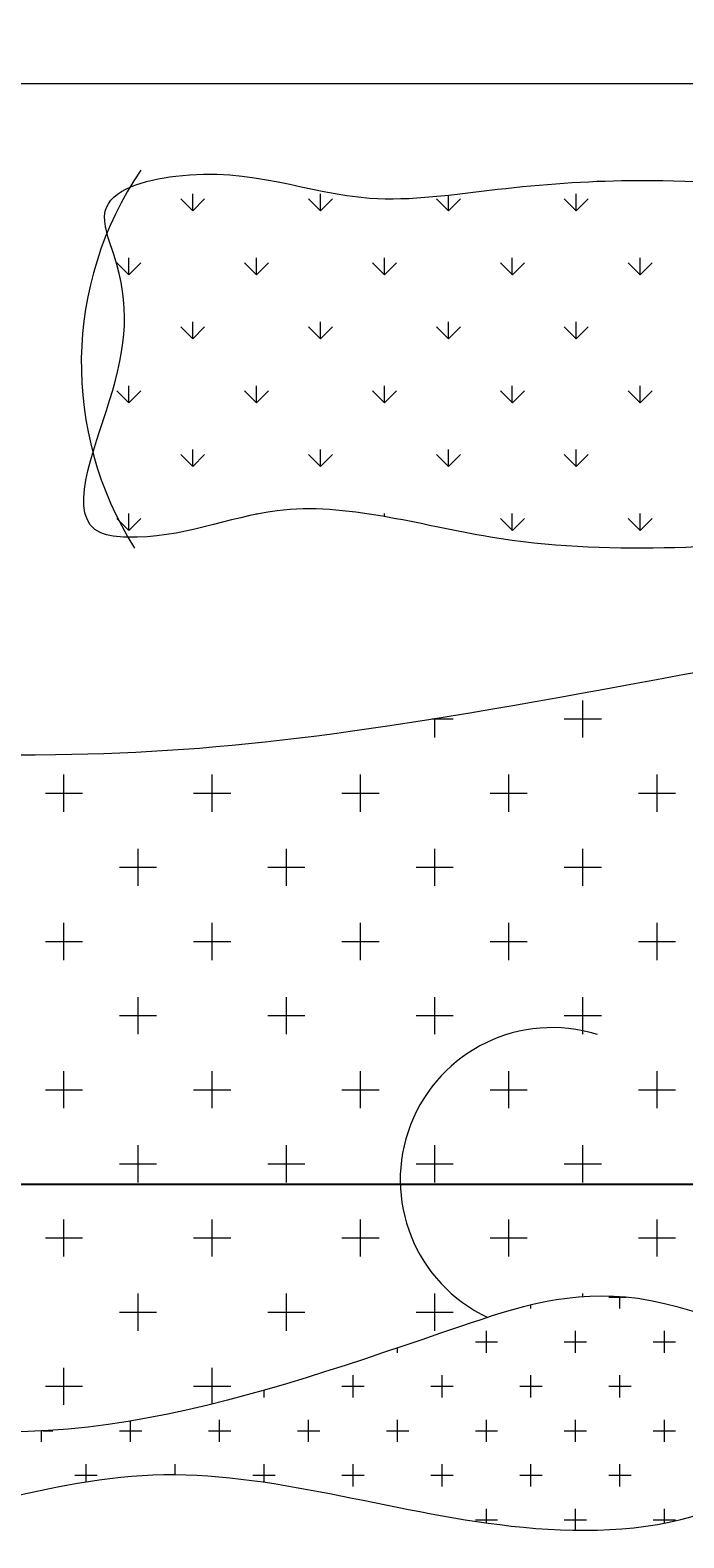
# Model space of a CAD drawing. Units: inches. Extents: x 2330 to 3943, y 1763 to 3461.
# Tile 6 of 40: x 2564 to 2593, y 2316 to 2383. Entities that reach past the tile are written whole.
import ezdxf

# ---------------------------------------------------------------- set-up
doc = ezdxf.new("R2010")
doc.units = ezdxf.units.IN
doc.layers.add('A-ANNO-DIMS', color=2, linetype='Continuous', lineweight=18)
doc.layers.add('A-FURN', color=8, linetype='Continuous', lineweight=13)
doc.styles.get("Standard").update_dxf_attribs({"font": 'arial.ttf'})
doc.dimstyles.get("Standard").update_dxf_attribs({"dimtxt": 0.18, "dimasz": 0.18, "dimexe": 0.18, "dimexo": 0.0625, "dimgap": 0.09, "dimtad": 0, "dimtih": 1, "dimtoh": 1, "dimdec": 4, "dimzin": 0, "dimdsep": 46, "dimtxsty": 'Standard', "dimcen": 0.09, "dimadec": 0, "dimazin": 0, "dimtfac": 1, "dimtdec": 4, "dimtofl": 0, "dimtmove": 0, "dimatfit": 3, "dimfxl": 1, "dimtolj": 1, "dimtzin": 0, "dimarcsym": 0})

# ---------------------------------------------------------------- blocks, each defined once
blk = doc.blocks.new('A$C200C7901')
for p, q in [((0.5, 2.3334), (2, 2.3334)), ((1.3176, 2.1721), (1.3075, 2.1822)), ((1.3176, 2.1721), (1.3075, 2.1822))]:
    blk.add_line(p, q)
at = {"linetype": 'ByBlock'}
for p, q in [((1.3714, 2.2259), (1.3714, 2.2402)), ((1.3714, 2.2259), (1.3714, 2.2402)), ((1.4792, 2.2259), (1.4792, 2.2402)), ((1.4792, 2.2259), (1.4792, 2.2402)), ((1.587, 2.2259), (1.587, 2.2393)), ((1.587, 2.2259), (1.587, 2.2393)), ((1.6947, 2.2259), (1.6947, 2.2402)), ((1.6947, 2.2259), (1.6947, 2.2402)), ((1.3714, 2.2259), (1.3613, 2.236)), ((1.3714, 2.2259), (1.3613, 2.236)), ((1.3714, 2.2259), (1.3815, 2.236)), ((1.3714, 2.2259), (1.3815, 2.236)), ((1.4792, 2.2259), (1.4691, 2.236)), ((1.4792, 2.2259), (1.4691, 2.236)), ((1.4792, 2.2259), (1.4893, 2.236)), ((1.4792, 2.2259), (1.4893, 2.236)), ((1.587, 2.2259), (1.5769, 2.236)), ((1.587, 2.2259), (1.5769, 2.236)), ((1.587, 2.2259), (1.5971, 2.236)), ((1.587, 2.2259), (1.5971, 2.236)), ((1.6947, 2.2259), (1.6846, 2.236)), ((1.6947, 2.2259), (1.6846, 2.236)), ((1.6947, 2.2259), (1.7048, 2.236)), ((1.6947, 2.2259), (1.7048, 2.236)), ((1.3176, 2.172), (1.3176, 2.1863)), ((1.3176, 2.172), (1.3176, 2.1863)), ((1.4253, 2.172), (1.4253, 2.1863)), ((1.4253, 2.172), (1.4253, 2.1863)), ((1.5331, 2.172), (1.5331, 2.1863)), ((1.5331, 2.172), (1.5331, 2.1863)), ((1.6408, 2.172), (1.6408, 2.1863)), ((1.6408, 2.172), (1.6408, 2.1863)), ((1.7486, 2.172), (1.7486, 2.1863)), ((1.7486, 2.172), (1.7486, 2.1863)), ((1.3176, 2.1721), (1.3277, 2.1822)), ((1.3176, 2.1721), (1.3277, 2.1822)), ((1.4253, 2.1721), (1.4152, 2.1822)), ((1.4253, 2.1721), (1.4152, 2.1822)), ((1.4253, 2.1721), (1.4354, 2.1822)), ((1.4253, 2.1721), (1.4354, 2.1822)), ((1.5331, 2.1721), (1.523, 2.1822)), ((1.5331, 2.1721), (1.523, 2.1822)), ((1.5331, 2.1721), (1.5432, 2.1822)), ((1.5331, 2.1721), (1.5432, 2.1822)), ((1.6409, 2.1721), (1.6308, 2.1822)), ((1.6409, 2.1721), (1.6308, 2.1822)), ((1.6409, 2.1721), (1.651, 2.1822)), ((1.6409, 2.1721), (1.651, 2.1822)), ((1.7486, 2.1721), (1.7385, 2.1822)), ((1.7486, 2.1721), (1.7385, 2.1822)), ((1.7486, 2.1721), (1.7587, 2.1822)), ((1.7486, 2.1721), (1.7587, 2.1822)), ((1.3714, 2.1182), (1.3613, 2.1283)), ((1.3714, 2.1182), (1.3613, 2.1283)), ((1.3714, 2.1182), (1.3714, 2.1325)), ((1.3714, 2.1182), (1.3714, 2.1325)), ((1.3714, 2.1182), (1.3815, 2.1283)), ((1.3714, 2.1182), (1.3815, 2.1283)), ((1.4792, 2.1182), (1.4691, 2.1283)), ((1.4792, 2.1182), (1.4691, 2.1283)), ((1.4792, 2.1182), (1.4792, 2.1325)), ((1.4792, 2.1182), (1.4792, 2.1325)), ((1.4792, 2.1182), (1.4893, 2.1283)), ((1.4792, 2.1182), (1.4893, 2.1283)), ((1.587, 2.1182), (1.5769, 2.1283)), ((1.587, 2.1182), (1.5769, 2.1283)), ((1.587, 2.1182), (1.587, 2.1325)), ((1.587, 2.1182), (1.587, 2.1325)), ((1.587, 2.1182), (1.5971, 2.1283)), ((1.587, 2.1182), (1.5971, 2.1283)), ((1.6947, 2.1182), (1.6846, 2.1283)), ((1.6947, 2.1182), (1.6846, 2.1283)), ((1.6947, 2.1182), (1.6947, 2.1325)), ((1.6947, 2.1182), (1.6947, 2.1325)), ((1.6947, 2.1182), (1.7048, 2.1283)), ((1.6947, 2.1182), (1.7048, 2.1283)), ((1.3176, 2.0643), (1.3075, 2.0744)), ((1.3176, 2.0643), (1.3075, 2.0744)), ((1.3176, 2.0643), (1.3176, 2.0786)), ((1.3176, 2.0643), (1.3176, 2.0786)), ((1.3176, 2.0643), (1.3277, 2.0744)), ((1.3176, 2.0643), (1.3277, 2.0744)), ((1.4253, 2.0643), (1.4152, 2.0744)), ((1.4253, 2.0643), (1.4152, 2.0744)), ((1.4253, 2.0643), (1.4253, 2.0786)), ((1.4253, 2.0643), (1.4253, 2.0786)), ((1.4253, 2.0643), (1.4354, 2.0744)), ((1.4253, 2.0643), (1.4354, 2.0744)), ((1.5331, 2.0643), (1.523, 2.0744)), ((1.5331, 2.0643), (1.523, 2.0744)), ((1.5331, 2.0643), (1.5331, 2.0786)), ((1.5331, 2.0643), (1.5331, 2.0786)), ((1.5331, 2.0643), (1.5432, 2.0744)), ((1.5331, 2.0643), (1.5432, 2.0744)), ((1.6409, 2.0643), (1.6308, 2.0744)), ((1.6409, 2.0643), (1.6308, 2.0744)), ((1.6408, 2.0643), (1.6408, 2.0786)), ((1.6408, 2.0643), (1.6408, 2.0786)), ((1.6409, 2.0643), (1.651, 2.0744)), ((1.6409, 2.0643), (1.651, 2.0744)), ((1.7486, 2.0643), (1.7385, 2.0744)), ((1.7486, 2.0643), (1.7385, 2.0744)), ((1.7486, 2.0643), (1.7486, 2.0786)), ((1.7486, 2.0643), (1.7486, 2.0786)), ((1.7486, 2.0643), (1.7587, 2.0744)), ((1.7486, 2.0643), (1.7587, 2.0744)), ((1.3714, 2.0104), (1.3714, 2.0247)), ((1.3714, 2.0104), (1.3714, 2.0247)), ((1.4792, 2.0104), (1.4792, 2.0247)), ((1.4792, 2.0104), (1.4792, 2.0247)), ((1.587, 2.0104), (1.587, 2.0247)), ((1.587, 2.0104), (1.587, 2.0247)), ((1.6947, 2.0104), (1.6947, 2.0247)), ((1.6947, 2.0104), (1.6947, 2.0247)), ((1.3714, 2.0104), (1.3613, 2.0205)), ((1.3714, 2.0104), (1.3613, 2.0205)), ((1.3714, 2.0104), (1.3815, 2.0205)), ((1.3714, 2.0104), (1.3815, 2.0205)), ((1.4792, 2.0104), (1.4691, 2.0205)), ((1.4792, 2.0104), (1.4691, 2.0205)), ((1.4792, 2.0104), (1.4893, 2.0205)), ((1.4792, 2.0104), (1.4893, 2.0205)), ((1.587, 2.0104), (1.5769, 2.0205)), ((1.587, 2.0104), (1.5769, 2.0205)), ((1.587, 2.0104), (1.5971, 2.0205)), ((1.587, 2.0104), (1.5971, 2.0205)), ((1.6947, 2.0104), (1.6846, 2.0205)), ((1.6947, 2.0104), (1.6846, 2.0205)), ((1.6947, 2.0104), (1.7048, 2.0205)), ((1.6947, 2.0104), (1.7048, 2.0205)), ((1.3176, 1.9565), (1.3176, 1.9708)), ((1.3176, 1.9565), (1.3176, 1.9708)), ((1.4253, 1.9703), (1.4253, 1.9708)), ((1.4253, 1.9703), (1.4253, 1.9708)), ((1.5331, 1.9683), (1.5331, 1.9708)), ((1.5331, 1.9683), (1.5331, 1.9708)), ((1.6408, 1.9565), (1.6408, 1.9708)), ((1.6408, 1.9565), (1.6408, 1.9708)), ((1.7486, 1.9565), (1.7486, 1.9708)), ((1.7486, 1.9565), (1.7486, 1.9708)), ((1.3176, 1.9565), (1.3075, 1.9666)), ((1.3176, 1.9565), (1.3075, 1.9666)), ((1.3176, 1.9565), (1.3277, 1.9666)), ((1.3176, 1.9565), (1.3277, 1.9666)), ((1.543, 1.9665), (1.5432, 1.9666)), ((1.543, 1.9665), (1.5432, 1.9666)), ((1.6409, 1.9565), (1.6308, 1.9666)), ((1.6409, 1.9565), (1.6308, 1.9666)), ((1.6409, 1.9565), (1.651, 1.9666)), ((1.6409, 1.9565), (1.651, 1.9666)), ((1.7486, 1.9565), (1.7385, 1.9666)), ((1.7486, 1.9565), (1.7385, 1.9666)), ((1.7486, 1.9565), (1.7587, 1.9666)), ((1.7486, 1.9565), (1.7587, 1.9666)), ((1.7004, 1.782), (1.7004, 1.8133)), ((1.7004, 1.782), (1.7004, 1.8133)), ((1.573, 1.7977), (1.591, 1.7977)), ((1.573, 1.7977), (1.591, 1.7977)), ((1.5754, 1.782), (1.5754, 1.7981)), ((1.5754, 1.782), (1.5754, 1.7981)), ((1.6847, 1.7977), (1.716, 1.7977)), ((1.6847, 1.7977), (1.716, 1.7977)), ((1.2629, 1.7195), (1.2629, 1.7508)), ((1.2629, 1.7195), (1.2629, 1.7508)), ((1.3879, 1.7195), (1.3879, 1.7508)), ((1.3879, 1.7195), (1.3879, 1.7508)), ((1.5129, 1.7195), (1.5129, 1.7508)), ((1.5129, 1.7195), (1.5129, 1.7508)), ((1.6379, 1.7195), (1.6379, 1.7508)), ((1.6379, 1.7195), (1.6379, 1.7508)), ((1.7629, 1.7195), (1.7629, 1.7508)), ((1.7629, 1.7195), (1.7629, 1.7508)), ((1.2472, 1.7352), (1.2785, 1.7352)), ((1.2472, 1.7352), (1.2785, 1.7352)), ((1.3722, 1.7352), (1.4035, 1.7352)), ((1.3722, 1.7352), (1.4035, 1.7352)), ((1.4972, 1.7352), (1.5285, 1.7352)), ((1.4972, 1.7352), (1.5285, 1.7352)), ((1.6222, 1.7352), (1.6535, 1.7352)), ((1.6222, 1.7352), (1.6535, 1.7352)), ((1.7472, 1.7352), (1.7785, 1.7352)), ((1.7472, 1.7352), (1.7785, 1.7352)), ((1.3254, 1.657), (1.3254, 1.6883)), ((1.3254, 1.657), (1.3254, 1.6883)), ((1.4504, 1.657), (1.4504, 1.6883)), ((1.4504, 1.657), (1.4504, 1.6883)), ((1.5754, 1.657), (1.5754, 1.6883)), ((1.5754, 1.657), (1.5754, 1.6883)), ((1.7004, 1.657), (1.7004, 1.6883)), ((1.7004, 1.657), (1.7004, 1.6883)), ((1.3097, 1.6727), (1.341, 1.6727)), ((1.3097, 1.6727), (1.341, 1.6727)), ((1.4347, 1.6727), (1.466, 1.6727)), ((1.4347, 1.6727), (1.466, 1.6727)), ((1.5597, 1.6727), (1.591, 1.6727)), ((1.5597, 1.6727), (1.591, 1.6727)), ((1.6847, 1.6727), (1.716, 1.6727)), ((1.6847, 1.6727), (1.716, 1.6727)), ((1.2629, 1.5945), (1.2629, 1.6258)), ((1.2629, 1.5945), (1.2629, 1.6258)), ((1.3879, 1.5945), (1.3879, 1.6258)), ((1.3879, 1.5945), (1.3879, 1.6258)), ((1.5129, 1.5945), (1.5129, 1.6258)), ((1.5129, 1.5945), (1.5129, 1.6258)), ((1.6379, 1.5945), (1.6379, 1.6258)), ((1.6379, 1.5945), (1.6379, 1.6258)), ((1.7629, 1.5945), (1.7629, 1.6258)), ((1.7629, 1.5945), (1.7629, 1.6258)), ((1.2472, 1.6102), (1.2785, 1.6102)), ((1.2472, 1.6102), (1.2785, 1.6102)), ((1.3722, 1.6102), (1.4035, 1.6102)), ((1.3722, 1.6102), (1.4035, 1.6102)), ((1.4972, 1.6102), (1.5285, 1.6102)), ((1.4972, 1.6102), (1.5285, 1.6102)), ((1.6222, 1.6102), (1.6535, 1.6102)), ((1.6222, 1.6102), (1.6535, 1.6102)), ((1.7472, 1.6102), (1.7785, 1.6102)), ((1.7472, 1.6102), (1.7785, 1.6102)), ((1.3254, 1.532), (1.3254, 1.5633)), ((1.3254, 1.532), (1.3254, 1.5633)), ((1.4504, 1.532), (1.4504, 1.5633)), ((1.4504, 1.532), (1.4504, 1.5633)), ((1.5754, 1.532), (1.5754, 1.5633)), ((1.5754, 1.532), (1.5754, 1.5633)), ((1.7004, 1.532), (1.7004, 1.5633)), ((1.7004, 1.532), (1.7004, 1.5633)), ((1.3097, 1.5477), (1.341, 1.5477)), ((1.3097, 1.5477), (1.341, 1.5477)), ((1.4347, 1.5477), (1.466, 1.5477)), ((1.4347, 1.5477), (1.466, 1.5477)), ((1.5597, 1.5477), (1.591, 1.5477)), ((1.5597, 1.5477), (1.591, 1.5477)), ((1.6847, 1.5477), (1.716, 1.5477)), ((1.6847, 1.5477), (1.716, 1.5477)), ((1.2629, 1.4695), (1.2629, 1.5008)), ((1.2629, 1.4695), (1.2629, 1.5008)), ((1.3879, 1.4695), (1.3879, 1.5008)), ((1.3879, 1.4695), (1.3879, 1.5008)), ((1.5129, 1.4695), (1.5129, 1.5008)), ((1.5129, 1.4695), (1.5129, 1.5008)), ((1.6379, 1.4695), (1.6379, 1.5008)), ((1.6379, 1.4695), (1.6379, 1.5008)), ((1.7629, 1.4695), (1.7629, 1.5008)), ((1.7629, 1.4695), (1.7629, 1.5008)), ((1.2472, 1.4852), (1.2785, 1.4852)), ((1.2472, 1.4852), (1.2785, 1.4852)), ((1.3722, 1.4852), (1.4035, 1.4852)), ((1.3722, 1.4852), (1.4035, 1.4852)), ((1.4972, 1.4852), (1.5285, 1.4852)), ((1.4972, 1.4852), (1.5285, 1.4852)), ((1.6222, 1.4852), (1.6535, 1.4852)), ((1.6222, 1.4852), (1.6535, 1.4852)), ((1.7472, 1.4852), (1.7785, 1.4852)), ((1.7472, 1.4852), (1.7785, 1.4852)), ((1.3254, 1.407), (1.3254, 1.4383)), ((1.3254, 1.407), (1.3254, 1.4383)), ((1.4504, 1.407), (1.4504, 1.4383)), ((1.4504, 1.407), (1.4504, 1.4383)), ((1.5754, 1.407), (1.5754, 1.4383)), ((1.5754, 1.407), (1.5754, 1.4383)), ((1.7004, 1.407), (1.7004, 1.4383)), ((1.7004, 1.407), (1.7004, 1.4383)), ((1.3097, 1.4227), (1.341, 1.4227)), ((1.3097, 1.4227), (1.341, 1.4227)), ((1.4347, 1.4227), (1.466, 1.4227)), ((1.4347, 1.4227), (1.466, 1.4227)), ((1.5597, 1.4227), (1.591, 1.4227)), ((1.5597, 1.4227), (1.591, 1.4227)), ((1.6847, 1.4227), (1.716, 1.4227)), ((1.6847, 1.4227), (1.716, 1.4227)), ((1.2629, 1.3445), (1.2629, 1.3758)), ((1.2629, 1.3445), (1.2629, 1.3758)), ((1.3879, 1.3445), (1.3879, 1.3758)), ((1.3879, 1.3445), (1.3879, 1.3758)), ((1.5129, 1.3445), (1.5129, 1.3758)), ((1.5129, 1.3445), (1.5129, 1.3758)), ((1.6379, 1.3445), (1.6379, 1.3758)), ((1.6379, 1.3445), (1.6379, 1.3758)), ((1.7629, 1.3445), (1.7629, 1.3758)), ((1.7629, 1.3445), (1.7629, 1.3758)), ((1.2472, 1.3602), (1.2785, 1.3602)), ((1.2472, 1.3602), (1.2785, 1.3602)), ((1.3722, 1.3602), (1.4035, 1.3602)), ((1.3722, 1.3602), (1.4035, 1.3602)), ((1.4972, 1.3602), (1.5285, 1.3602)), ((1.4972, 1.3602), (1.5285, 1.3602)), ((1.6222, 1.3602), (1.6535, 1.3602)), ((1.6222, 1.3602), (1.6535, 1.3602)), ((1.7472, 1.3602), (1.7785, 1.3602)), ((1.7472, 1.3602), (1.7785, 1.3602)), ((1.3254, 1.282), (1.3254, 1.3133)), ((1.3254, 1.282), (1.3254, 1.3133)), ((1.4504, 1.282), (1.4504, 1.3133)), ((1.4504, 1.282), (1.4504, 1.3133)), ((1.5754, 1.282), (1.5754, 1.3133)), ((1.5754, 1.282), (1.5754, 1.3133)), ((1.7004, 1.3106), (1.7004, 1.3133)), ((1.7004, 1.3106), (1.7004, 1.3133)), ((1.7222, 1.3102), (1.7369, 1.3102)), ((1.7222, 1.3102), (1.7369, 1.3102)), ((1.7316, 1.3008), (1.7316, 1.3106)), ((1.7316, 1.3008), (1.7316, 1.3106)), ((1.3097, 1.2977), (1.341, 1.2977)), ((1.3097, 1.2977), (1.341, 1.2977)), ((1.4347, 1.2977), (1.466, 1.2977)), ((1.4347, 1.2977), (1.466, 1.2977)), ((1.5597, 1.2977), (1.591, 1.2977)), ((1.5597, 1.2977), (1.591, 1.2977)), ((1.6566, 1.3008), (1.6566, 1.3036)), ((1.6566, 1.3008), (1.6566, 1.3036)), ((1.6097, 1.2727), (1.6285, 1.2727)), ((1.6097, 1.2727), (1.6285, 1.2727)), ((1.6191, 1.2633), (1.6191, 1.282)), ((1.6191, 1.2633), (1.6191, 1.282)), ((1.6847, 1.2727), (1.7035, 1.2727)), ((1.6847, 1.2727), (1.7035, 1.2727)), ((1.6941, 1.2633), (1.6941, 1.282)), ((1.6941, 1.2633), (1.6941, 1.282)), ((1.7597, 1.2727), (1.7785, 1.2727)), ((1.7597, 1.2727), (1.7785, 1.2727)), ((1.7691, 1.2633), (1.7691, 1.282)), ((1.7691, 1.2633), (1.7691, 1.282)), ((1.5441, 1.2633), (1.5441, 1.2675)), ((1.5441, 1.2633), (1.5441, 1.2675)), ((1.2629, 1.2195), (1.2629, 1.2508)), ((1.2629, 1.2195), (1.2629, 1.2508)), ((1.3879, 1.2202), (1.3879, 1.2508)), ((1.3879, 1.2202), (1.3879, 1.2508)), ((1.2472, 1.2352), (1.2785, 1.2352)), ((1.2472, 1.2352), (1.2785, 1.2352)), ((1.3722, 1.2352), (1.4035, 1.2352)), ((1.3722, 1.2352), (1.4035, 1.2352)), ((1.4972, 1.2352), (1.516, 1.2352)), ((1.4972, 1.2352), (1.516, 1.2352)), ((1.5066, 1.2258), (1.5066, 1.2445)), ((1.5066, 1.2258), (1.5066, 1.2445)), ((1.5722, 1.2352), (1.591, 1.2352)), ((1.5722, 1.2352), (1.591, 1.2352)), ((1.5816, 1.2258), (1.5816, 1.2445)), ((1.5816, 1.2258), (1.5816, 1.2445)), ((1.6472, 1.2352), (1.666, 1.2352)), ((1.6472, 1.2352), (1.666, 1.2352)), ((1.6566, 1.2258), (1.6566, 1.2445)), ((1.6566, 1.2258), (1.6566, 1.2445)), ((1.7222, 1.2352), (1.741, 1.2352)), ((1.7222, 1.2352), (1.741, 1.2352)), ((1.7316, 1.2258), (1.7316, 1.2445)), ((1.7316, 1.2258), (1.7316, 1.2445)), ((1.4316, 1.2258), (1.4316, 1.2318)), ((1.4316, 1.2258), (1.4316, 1.2318)), ((1.2441, 1.1883), (1.2441, 1.1976)), ((1.2441, 1.1883), (1.2441, 1.1976)), ((1.2452, 1.1977), (1.2535, 1.1977)), ((1.2452, 1.1977), (1.2535, 1.1977)), ((1.3097, 1.1977), (1.3285, 1.1977)), ((1.3097, 1.1977), (1.3285, 1.1977)), ((1.3191, 1.1883), (1.3191, 1.2059)), ((1.3191, 1.1883), (1.3191, 1.2059)), ((1.3847, 1.1977), (1.4035, 1.1977)), ((1.3847, 1.1977), (1.4035, 1.1977)), ((1.3941, 1.1883), (1.3941, 1.207)), ((1.3941, 1.1883), (1.3941, 1.207)), ((1.4597, 1.1977), (1.4785, 1.1977)), ((1.4597, 1.1977), (1.4785, 1.1977)), ((1.4691, 1.1883), (1.4691, 1.207)), ((1.4691, 1.1883), (1.4691, 1.207)), ((1.5347, 1.1977), (1.5535, 1.1977)), ((1.5347, 1.1977), (1.5535, 1.1977)), ((1.5441, 1.1883), (1.5441, 1.207)), ((1.5441, 1.1883), (1.5441, 1.207)), ((1.6097, 1.1977), (1.6285, 1.1977)), ((1.6097, 1.1977), (1.6285, 1.1977)), ((1.6191, 1.1883), (1.6191, 1.207)), ((1.6191, 1.1883), (1.6191, 1.207)), ((1.6847, 1.1977), (1.7035, 1.1977)), ((1.6847, 1.1977), (1.7035, 1.1977)), ((1.6941, 1.1883), (1.6941, 1.207)), ((1.6941, 1.1883), (1.6941, 1.207)), ((1.7597, 1.1977), (1.7785, 1.1977)), ((1.7597, 1.1977), (1.7785, 1.1977)), ((1.7691, 1.1883), (1.7691, 1.207)), ((1.7691, 1.1883), (1.7691, 1.207)), ((1.2816, 1.1547), (1.2816, 1.1695)), ((1.2816, 1.1547), (1.2816, 1.1695)), ((1.3566, 1.1608), (1.3566, 1.1695)), ((1.3566, 1.1608), (1.3566, 1.1695)), ((1.4316, 1.1544), (1.4316, 1.1695)), ((1.4316, 1.1544), (1.4316, 1.1695)), ((1.5066, 1.1508), (1.5066, 1.1695)), ((1.5066, 1.1508), (1.5066, 1.1695)), ((1.5816, 1.1508), (1.5816, 1.1695)), ((1.5816, 1.1508), (1.5816, 1.1695)), ((1.6566, 1.1508), (1.6566, 1.1695)), ((1.6566, 1.1508), (1.6566, 1.1695)), ((1.7316, 1.1508), (1.7316, 1.1695)), ((1.7316, 1.1508), (1.7316, 1.1695)), ((1.2722, 1.1602), (1.291, 1.1602)), ((1.2722, 1.1602), (1.291, 1.1602)), ((1.4222, 1.1602), (1.441, 1.1602)), ((1.4222, 1.1602), (1.441, 1.1602)), ((1.4972, 1.1602), (1.516, 1.1602)), ((1.4972, 1.1602), (1.516, 1.1602)), ((1.5722, 1.1602), (1.591, 1.1602)), ((1.5722, 1.1602), (1.591, 1.1602)), ((1.6472, 1.1602), (1.666, 1.1602)), ((1.6472, 1.1602), (1.666, 1.1602)), ((1.7222, 1.1602), (1.741, 1.1602)), ((1.7222, 1.1602), (1.741, 1.1602)), ((1.6191, 1.1201), (1.6191, 1.132)), ((1.6191, 1.1201), (1.6191, 1.132)), ((1.6941, 1.1139), (1.6941, 1.132)), ((1.6941, 1.1139), (1.6941, 1.132)), ((1.7691, 1.1198), (1.7691, 1.132)), ((1.7691, 1.1198), (1.7691, 1.132)), ((1.6097, 1.1227), (1.6285, 1.1227)), ((1.6097, 1.1227), (1.6285, 1.1227)), ((1.6847, 1.1227), (1.7035, 1.1227)), ((1.6847, 1.1227), (1.7035, 1.1227)), ((1.7597, 1.1227), (1.7785, 1.1227)), ((1.7597, 1.1227), (1.7785, 1.1227))]:
    blk.add_line(p, q, dxfattribs=at)
blk.add_arc((1.5685, 2.097), 0.291, 145.8603, 212.2445)
blk.add_arc((1.6746, 1.4093), 0.1282, 72.7909, 244.8695, dxfattribs=at)
blk.add_arc((1.6746, 1.4093), 0.1282, 72.7909, 244.8695, dxfattribs=at)
for points, knots in [([(1.9146, 1.951), (1.8174, 1.9428), (1.6601, 1.9297), (1.4574, 1.9942), (1.3549, 1.9462), (1.2593, 1.9563), (1.314, 2.0834), (1.3193, 2.1569), (1.2853, 2.2393), (1.4031, 2.2724), (1.4987, 2.2256), (1.6304, 2.2459), (1.7519, 2.2548), (1.8574, 2.2473), (1.9254, 2.2478), (1.9438, 2.2479)], [0, 0, 0, 0, 292.165466, 473.33038, 601.631673, 624.236147, 735.870502, 858.452188, 896.317728, 962.783971, 1127.3494, 1235.376134, 1347.110578, 1495.806953, 1551.11062, 1551.11062, 1551.11062, 1551.11062]), ([(0.4485, 1.7835), (0.4321, 1.7496), (0.4062, 1.6964), (0.49, 1.6713), (0.4719, 1.5969), (0.4123, 1.592), (0.4233, 1.5337), (0.4954, 1.5086), (0.4012, 1.4738), (0.3253, 1.4306), (0.4113, 1.3764), (0.3688, 1.3065), (0.5579, 1.2663), (0.741, 1.4533), (1.1127, 1.1109), (1.4811, 1.2478), (1.7885, 1.3492), (2.0357, 1.1637), (2.0748, 1.2974), (2.0876, 1.349), (2.0192, 1.3805), (2.0564, 1.4298), (2.0588, 1.4846), (1.9759, 1.5349), (2.1004, 1.5845), (2.0397, 1.6519), (1.971, 1.7053), (2.1104, 1.8981), (1.5946, 1.7967), (1.2448, 1.7472), (0.8129, 1.7935), (0.4953, 1.8548), (0.4582, 1.7983), (0.4485, 1.7835)], [0, 0, 0, 0, 88.420092, 139.08588, 204.302936, 239.695496, 287.801042, 327.365471, 412.960499, 463.626286, 552.059846, 584.668336, 662.614915, 940.993281, 1309.926334, 1844.022653, 1996.276242, 2316.43048, 2341.441004, 2404.707416, 2449.463774, 2514.680778, 2538.40571, 2613.031547, 2697.13096, 2760.903931, 2822.692699, 2945.47, 3215.060018, 3725.584917, 4361.974444, 4504.671998, 4555.32777, 4555.32777, 4555.32777, 4555.32777]), ([(0.4856, 1.3429), (0.5504, 1.3182), (0.6715, 1.2721), (0.8374, 1.0498), (1.1164, 1.1183), (1.3878, 1.1816), (1.5888, 1.1102), (1.8403, 1.1127), (1.9415, 1.2178), (2.0032, 1.2819)], [0, 0, 0, 0, 205.411753, 383.654933, 772.067458, 921.644661, 1226.793228, 1388.983508, 1642.292305, 1642.292305, 1642.292305, 1642.292305])]:
    blk.add_open_spline(points, degree=3, knots=knots)
blk.add_open_spline([(0.473, 1.2954), (0.4739, 1.2781), (0.4755, 1.2477), (0.5032, 1.2084), (0.4801, 1.1701), (0.4928, 1.1255), (0.4674, 1.0912), (0.4579, 1.0351), (0.501, 0.9724), (0.4311, 0.8832), (0.4902, 0.8637), (0.4843, 0.8288), (0.4774, 0.7906), (0.4625, 0.7457), (0.459, 0.6999), (0.4816, 0.6664), (0.4748, 0.625), (0.4791, 0.5889), (0.4533, 0.5528), (0.4738, 0.5004), (0.4658, 0.4502), (0.4696, 0.3946), (0.4189, 0.3935), (0.4493, 0.3684), (0.4694, 0.3857), (0.4922, 0.3576), (0.5297, 0.3262), (0.5917, 0.3353), (0.6454, 0.3754), (0.7083, 0.3741), (0.7643, 0.3328), (0.826, 0.346), (0.925, 0.3388), (1.0353, 0.3593), (1.1561, 0.3744), (1.2477, 0.3154), (1.3302, 0.3474), (1.4086, 0.3512), (1.5217, 0.3878), (1.6362, 0.3176), (1.7682, 0.3285), (1.8402, 0.3019), (1.9071, 0.3529), (1.9647, 0.3412), (2.0795, 0.2948), (2.0472, 0.3498), (2.0343, 0.3772), (2.0435, 0.43), (2.0109, 0.5782), (2.0746, 0.4643), (2.0805, 0.584), (2.0084, 0.5979), (2.0343, 0.6846), (2.0344, 0.746), (2.0293, 0.8096), (2.0489, 0.8545), (2.0652, 0.9218), (1.9842, 0.9297), (2.0007, 1.0162), (2.0367, 1.0585), (2.0367, 1.1102), (2.0457, 1.1647), (2.0226, 1.2084), (2.0234, 1.2306), (2.0236, 1.2352)], degree=3, knots=[0, 0, 0, 0, 51.660678, 90.967412, 128.902454, 170.303599, 219.852997, 247.834962, 336.321557, 429.35469, 458.821847, 477.222321, 524.135809, 581.038434, 617.839381, 657.146115, 693.947125, 740.178081, 760.753248, 820.731705, 885.133458, 928.777044, 953.563729, 976.574207, 995.553042, 1018.563482, 1064.584401, 1147.951297, 1174.787598, 1266.851571, 1308.018447, 1377.066427, 1441.511314, 1608.245014, 1714.11869, 1792.771707, 1913.247991, 1954.931389, 2029.864445, 2259.189419, 2305.221512, 2429.507982, 2456.344283, 2543.92595, 2627.925037, 2662.96218, 2687.736879, 2719.937755, 2839.540991, 2875.47895, 2953.681041, 2993.270313, 3066.872333, 3154.395764, 3200.397042, 3248.426375, 3312.828127, 3347.881398, 3444.484026, 3481.577522, 3518.665244, 3592.267265, 3644.719162, 3658.519501, 3658.519501, 3658.519501, 3658.519501], dxfattribs=at)
blk = doc.blocks.new('*D39')
at = {"layer": 'A-ANNO-DIMS', "color": 0, "lineweight": -2, "transparency": 16777216}
for p, q in [((2499.499, 2380.496), (2499.499, 2400.343)), ((2499.679, 2400.163), (2563.823, 2400.163)), ((2630.845, 2400.163), (2566.701, 2400.163)), ((2631.025, 2380.496), (2631.025, 2400.343))]:
    blk.add_line(p, q, dxfattribs=at)
at = {"layer": 'A-ANNO-DIMS', "color": 0, "transparency": 16777216}
for points in [[(2499.679, 2400.193), (2499.679, 2400.133), (2499.499, 2400.163)], [(2630.845, 2400.193), (2630.845, 2400.133), (2631.025, 2400.163)]]:
    blk.add_solid(points, dxfattribs=at)
at = {"layer": 'Defpoints', "color": 0, "transparency": 16777216}
for p in [(2631.025, 2400.163), (2499.499, 2380.434), (2631.025, 2380.434)]:
    blk.add_point(p, dxfattribs=at)
at = {"layer": 'A-ANNO-DIMS', "color": 0, "transparency": 16777216, "insert": (2565.262, 2400.163), "char_height": 0.18, "attachment_point": 5}
blk.add_mtext('\\A1;DOUBLE BED 132 TYP.', dxfattribs=at)
blk = doc.blocks.new('*D80')
at = {"layer": 'A-ANNO-DIMS', "color": 0, "lineweight": -2, "transparency": 16777216}
for p, q in [((3166.598, 2331.698), (2330.502, 2331.698)), ((2330.682, 2331.518), (2330.682, 2322.357)), ((2330.682, 2312.832), (2330.682, 2321.993)), ((3166.598, 2312.652), (2330.502, 2312.652))]:
    blk.add_line(p, q, dxfattribs=at)
at = {"layer": 'A-ANNO-DIMS', "color": 0, "transparency": 16777216}
for points in [[(2330.652, 2331.518), (2330.712, 2331.518), (2330.682, 2331.698)], [(2330.652, 2312.832), (2330.712, 2312.832), (2330.682, 2312.652)]]:
    blk.add_solid(points, dxfattribs=at)
at = {"layer": 'Defpoints', "color": 0, "transparency": 16777216}
for p in [(2330.682, 2331.698), (3166.661, 2331.698), (3166.661, 2312.652)]:
    blk.add_point(p, dxfattribs=at)
at = {"layer": 'A-ANNO-DIMS', "color": 0, "transparency": 16777216, "insert": (2330.682, 2322.175), "char_height": 0.18, "attachment_point": 5}
blk.add_mtext('\\A1;19.046', dxfattribs=at)

msp = doc.modelspace()

# ---------------------------------------------------------------- block references
at = {"layer": 'A-FURN', "xscale": 52.5181391560459, "yscale": 52.5181391560459, "zscale": 52.5181391560459}
msp.add_blockref('A$C200C7901', (2499.4987, 2257.8888), dxfattribs=at)

# ---------------------------------------------------------------- dimensions: what is measured, and where the dimension line sits
at = {"layer": 'A-ANNO-DIMS'}
dim = msp.add_linear_dim(base=(2631.0254, 2400.1629), p1=(2499.4986, 2380.4339), p2=(2631.0254, 2380.4339), text='DOUBLE BED <> TYP.', dimstyle='Standard', override={"dimdec": 0, "dimlfac": 1, "dimrnd": 0, "dimzin": 0, "dimdsep": 46, "dimlunit": 2}, dxfattribs=at)
dim.commit()
dim.dimension.update_dxf_attribs({"geometry": '*D39', "text_midpoint": (2565.262, 2400.1629)})
dim = msp.add_linear_dim(base=(2330.6824, 2331.6982), p1=(3166.6605, 2312.6524), p2=(3166.6605, 2331.6982), angle=90, dimstyle='Standard', override={"dimdec": 3, "dimlfac": 1, "dimrnd": 0, "dimzin": 0, "dimdsep": 46, "dimlunit": 2}, dxfattribs=at)
dim.commit()
dim.dimension.update_dxf_attribs({"geometry": '*D80', "text_midpoint": (2330.6824, 2322.1753)})

doc.saveas('drawing.dxf')
